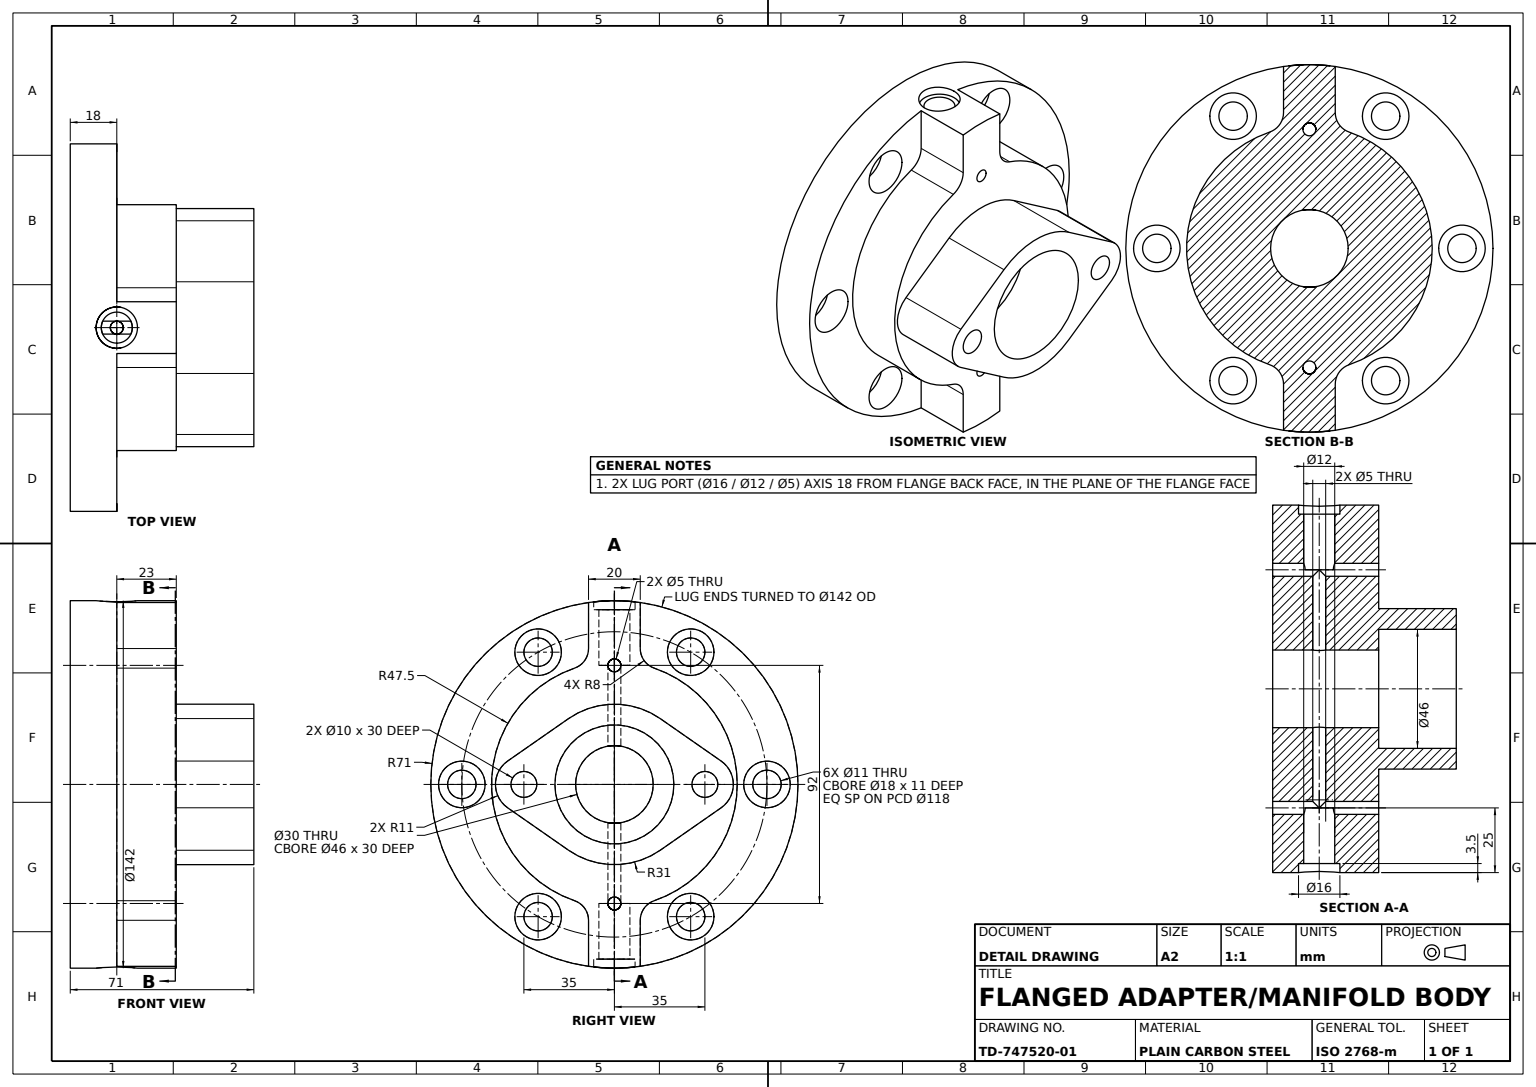
SolidWorks part; units mm, degrees
material "Plain Carbon Steel"
ref_plane "Front Plane" through (0, 0, 0) normal (0, 0, 1) x (1, 0, 0)
ref_plane "Top Plane" through (0, 0, 0) normal (0, 1, 0) x (1, 0, 0)
ref_plane "Right Plane" through (0, 0, 0) normal (1, 0, 0) x (0, 0, -1)
sketch "Base Flange Sketch" plane through (0, 0, 0) normal (0, 1, 0) x (1, 0, 0)
  circle A0 centre (0, 0) radius 71
  circle A2 centre (0, 59) radius 5.5
  circle A3 centre (51.0955, 29.5) radius 5.5
  circle A4 centre (51.0955, -29.5) radius 5.5
  circle A5 centre (0, -59) radius 5.5
  circle A6 centre (-51.0955, -29.5) radius 5.5
  circle A7 centre (-51.0955, 29.5) radius 5.5
  dimension "D1" = 142
  dimension "D2" = 59
  dimension "D3" = 11
  dimension "D5" = 29.5
  dimension "D6" = 51.0955
  dimension "D4" = 6
extrude "Base Flange Ø142 6xØ11" add sketch "Base Flange Sketch" along normal blind 18
sketch "Flange Counterbore Sketch" plane through (0, 18, 0) normal (0, 1, 0) x (1, 0, 0)
  circle A0 centre (0, 59) radius 9
  circle A1 centre (51.0955, 29.5) radius 9
  circle A2 centre (51.0955, -29.5) radius 9
  circle A3 centre (0, -59) radius 9
  circle A4 centre (-51.0955, -29.5) radius 9
  circle A5 centre (-51.0955, 29.5) radius 9
  dimension "D1" = 18
  dimension "D3" = 29.5
  dimension "D4" = 51.0955
  dimension "D2" = 6
extrude "Flange Counterbores 6xØ18" cut sketch "Flange Counterbore Sketch" against normal blind 11
sketch "Hub Sketch" plane through (0, 18, 0) normal (0, 1, 0) x (1, 0, 0)
  line L0 (52.5, 10) -> (70.2922, 10)
  line L1 (-70.2922, -10) -> (-52.5, -10)
  line L2 (-70.2922, 10) -> (-52.5, 10)
  line L3 (52.5, -10) -> (70.2922, -10)
  arc A1 (-44.9324, -15.4054) -> (44.9324, -15.4054) centre (0, 0) ccw
  arc A2 (-44.9324, -15.4054) -> (-52.5, -10) centre (-52.5, -18) ccw
  arc A3 (-70.2922, 10) -> (-70.2922, -10) centre (0, 0) ccw
  arc A4 (70.2922, -10) -> (70.2922, 10) centre (0, 0) ccw
  arc A5 (44.9324, 15.4054) -> (-44.9324, 15.4054) centre (0, 0) ccw
  arc A6 (44.9324, -15.4054) -> (52.5, -10) centre (52.5, -18) cw
  arc A7 (44.9324, 15.4054) -> (52.5, 10) centre (52.5, 18) ccw
  arc A8 (-52.5, 10) -> (-44.9324, 15.4054) centre (-52.5, 18) ccw
  point P3 (-71, 0)
  point P5 (71, 0)
  point P9 (-71, -10)
  point P10 (71, -10)
  point P11 (-71, 10)
  point P12 (71, 10)
  point P19 (46.4354, -10)
  point P23 (46.4354, 10)
  dimension "D1" = 95
  dimension "D4" = 142
  dimension "D2" = 8
  dimension "D5" = 70.2922
  dimension "D3" = 44.9324
  dimension "D6" = 17.7922
  dimension "D7" = 17.7922
extrude "Hub Ø95 with Side Lugs" add sketch "Hub Sketch" along normal blind 23
sketch "Lobed Cap Sketch" plane through (0, 41, 0) normal (0, 1, 0) x (1, 0, 0)
  line L0 (-25.4402, 17.7143) -> (-9.0272, 41.2857)
  line L1 (25.4402, 17.7143) -> (9.0272, 41.2857)
  line L2 (-25.4402, -17.7143) -> (-9.0272, -41.2857)
  line L3 (9.0272, -41.2857) -> (25.4402, -17.7143)
  arc A0 (9.0272, 41.2857) -> (-9.0272, 41.2857) centre (0, 35) ccw
  circle A1 centre (0, 35) radius 5
  arc A2 (-9.0272, -41.2857) -> (9.0272, -41.2857) centre (0, -35) ccw
  circle A3 centre (0, -35) radius 5
  arc A4 (-25.4402, 17.7143) -> (-25.4402, -17.7143) centre (0, 0) ccw
  circle A5 centre (0, 0) radius 23
  arc A6 (25.4402, -17.7143) -> (25.4402, 17.7143) centre (0, 0) ccw
  dimension "D1" = 22
  dimension "D2" = 10
  dimension "D3" = 22
  dimension "D4" = 10
  dimension "D9" = 62
  dimension "D10" = 46
  dimension "D5" = 35
  dimension "D6" = 35
  dimension "D7" = 52.5
  dimension "D8" = 52.5
extrude "Lobed Cap Boss" add sketch "Lobed Cap Sketch" along normal blind 30
sketch "Cap Holes Sketch" plane through (0, 41, 0) normal (0, 1, 0) x (1, 0, 0)
  circle A0 centre (-46, 0) radius 2.5
  circle A1 centre (46, 0) radius 2.5
  dimension "D1" = 5
  dimension "D2" = 5
  dimension "D3" = 46
  dimension "D4" = 46
  dimension "D5" = 92
extrude "Cap Holes 2xØ5" cut sketch "Cap Holes Sketch" against normal blind 60
sketch "Bore Sketch" plane through (0, 71, 0) normal (0, 1, 0) x (1, 0, 0)
  circle A2 centre (0, 0) radius 15
  dimension "D1" = 30
extrude "Bore Ø30" cut sketch "Bore Sketch" against normal up to surface (71 mm away) up to face at (-46, 0, 2.5)
ref_plane "Plane1" through (71, 0, 0) normal (1, 0, 0) x (0, 0, -1)
sketch "Cross Hole Sketch" plane through (71, 0, 0) normal (1, 0, 0) x (0, 0, -1)
  line L0 (71, 18) -> (10, 18) construction
  circle A0 centre (0, 18) radius 2.5
  dimension "D1" = 5
  dimension "D2" = 0
extrude "Cross Hole Ø5" cut sketch "Cross Hole Sketch" against normal blind 200
sketch "Side A Counterbore Sketch" plane through (71, 0, 0) normal (1, 0, 0) x (0, 0, -1)
  circle A0 centre (0, 18) radius 6
  dimension "D1" = 12
extrude "Side A Counterbore Ø12" cut sketch "Side A Counterbore Sketch" against normal blind 25
sketch "Side A Spotface Sketch" plane through (71, 0, 0) normal (1, 0, 0) x (0, 0, -1)
  circle A0 centre (0, 18) radius 8
  dimension "D1" = 16
extrude "Side A Spotface Ø16" cut sketch "Side A Spotface Sketch" against normal blind 3.5
ref_plane "Plane2" through (-71, 0, 0) normal (1, 0, 0) x (0, 0, -1)
sketch "Side B Counterbore Sketch" plane through (-71, 0, 0) normal (1, 0, 0) x (0, 0, -1)
  circle A0 centre (0, 18) radius 6
  dimension "D1" = 12
extrude "Side B Counterbore Ø12" cut sketch "Side B Counterbore Sketch" along normal blind 25
sketch "Side B Spotface Sketch" plane through (-71, 0, 0) normal (1, 0, 0) x (0, 0, -1)
  circle A0 centre (0, 18) radius 8
  dimension "D1" = 16
extrude "Side B Spotface Ø16" cut sketch "Side B Spotface Sketch" along normal blind 3.5
